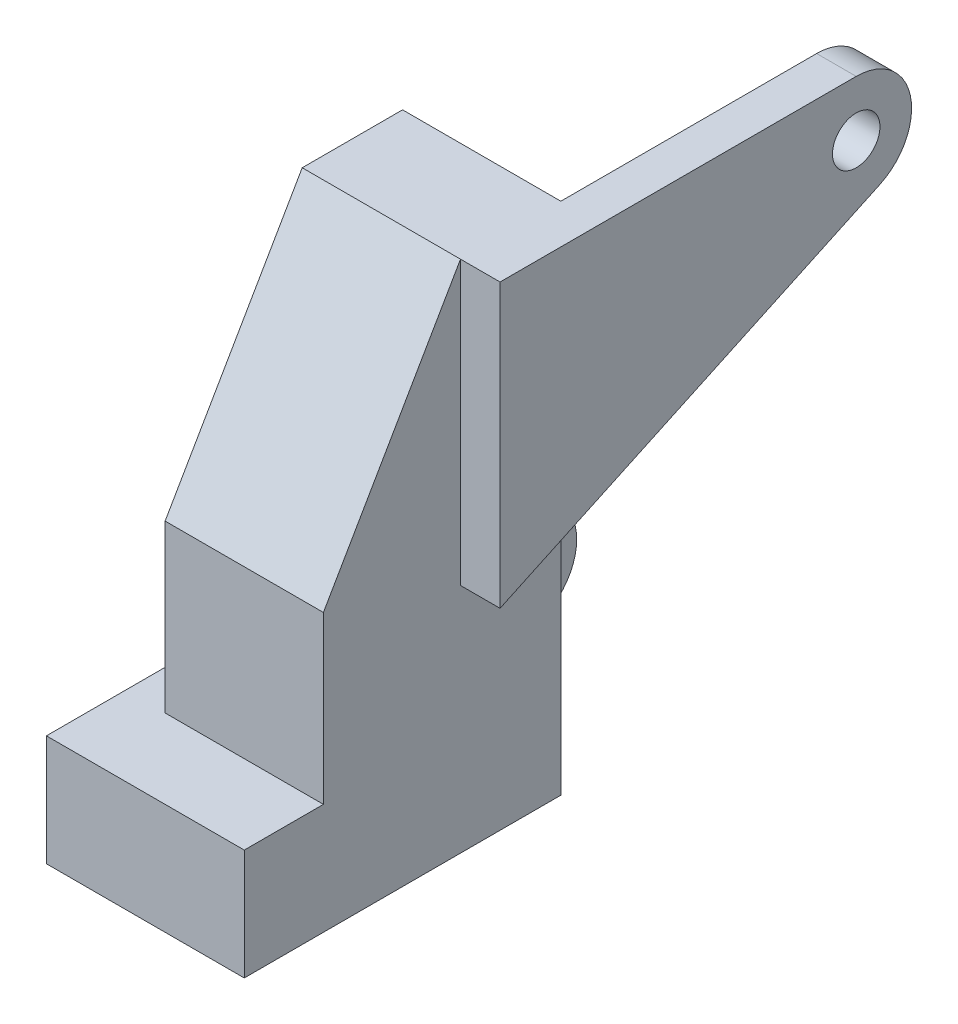
ISO-10303-21;
HEADER;
FILE_DESCRIPTION(('STEP AP214'),'2;1');
FILE_NAME('part.step','',(''),(''),'','','');
FILE_SCHEMA(('AUTOMOTIVE_DESIGN { 1 0 10303 214 1 1 1 1 }'));
ENDSEC;
DATA;
#1=APPLICATION_CONTEXT('core data for automotive mechanical design processes');
#2=APPLICATION_PROTOCOL_DEFINITION('international standard','automotive_design',2000,#1);
#3=PRODUCT_CONTEXT('',#1,'mechanical');
#4=PRODUCT('Part','Part','',(#3));
#5=PRODUCT_RELATED_PRODUCT_CATEGORY('part','',(#4));
#6=PRODUCT_DEFINITION_FORMATION('','',#4);
#7=PRODUCT_DEFINITION_CONTEXT('part definition',#1,'design');
#8=PRODUCT_DEFINITION('design','',#6,#7);
#9=PRODUCT_DEFINITION_SHAPE('','',#8);
#10=(LENGTH_UNIT() NAMED_UNIT(*) SI_UNIT(.MILLI.,.METRE.));
#11=(NAMED_UNIT(*) PLANE_ANGLE_UNIT() SI_UNIT($,.RADIAN.));
#12=(NAMED_UNIT(*) SI_UNIT($,.STERADIAN.) SOLID_ANGLE_UNIT());
#13=UNCERTAINTY_MEASURE_WITH_UNIT(LENGTH_MEASURE(1.E-05),#10,'distance_accuracy_value','');
#14=(GEOMETRIC_REPRESENTATION_CONTEXT(3) GLOBAL_UNCERTAINTY_ASSIGNED_CONTEXT((#13)) GLOBAL_UNIT_ASSIGNED_CONTEXT((#10,
#11,#12)) REPRESENTATION_CONTEXT('',''));
#15=CARTESIAN_POINT('',(0.,0.,0.));
#16=DIRECTION('',(0.,0.,1.));
#17=DIRECTION('',(1.,0.,0.));
#18=AXIS2_PLACEMENT_3D('',#15,#16,#17);
#19=CARTESIAN_POINT('',(9.99999999999999,32.5,40.));
#20=DIRECTION('',(-1.,0.,0.));
#21=DIRECTION('',(0.,-1.,0.));
#22=AXIS2_PLACEMENT_3D('',#19,#20,#21);
#23=PLANE('',#22);
#24=DIRECTION('',(0.,0.422618261740704,-0.906307787036648));
#25=VECTOR('',#24,1.);
#26=CARTESIAN_POINT('',(10.,-3.20749004971267,12.6794919243115));
#27=LINE('',#26,#25);
#28=CARTESIAN_POINT('',(10.,-3.20749004971267,12.6794919243115));
#29=VERTEX_POINT('',#28);
#30=CARTESIAN_POINT('',(10.,2.7050541361083,0.));
#31=VERTEX_POINT('',#30);
#32=EDGE_CURVE('E483',#29,#31,#27,.T.);
#33=ORIENTED_EDGE('',*,*,#32,.F.);
#34=DIRECTION('',(0.,-1.,0.));
#35=VECTOR('',#34,1.);
#36=CARTESIAN_POINT('',(9.99999999999999,32.5,12.6794919243115));
#37=LINE('',#36,#35);
#38=CARTESIAN_POINT('',(9.99999999999999,32.5,12.6794919243115));
#39=VERTEX_POINT('',#38);
#40=EDGE_CURVE('E481',#39,#29,#37,.T.);
#41=ORIENTED_EDGE('',*,*,#40,.F.);
#42=DIRECTION('',(0.,0.866025403784442,-0.499999999999995));
#43=VECTOR('',#42,1.);
#44=CARTESIAN_POINT('',(9.99999999999999,32.5,12.6794919243115));
#45=LINE('',#44,#43);
#46=CARTESIAN_POINT('',(10.,2.5,30.));
#47=VERTEX_POINT('',#46);
#48=EDGE_CURVE('E208',#47,#39,#45,.T.);
#49=ORIENTED_EDGE('',*,*,#48,.F.);
#50=DIRECTION('',(0.,1.,0.));
#51=VECTOR('',#50,1.);
#52=CARTESIAN_POINT('',(10.,-18.5,30.));
#53=LINE('',#52,#51);
#54=CARTESIAN_POINT('',(10.,-18.5,30.));
#55=VERTEX_POINT('',#54);
#56=EDGE_CURVE('E204',#55,#47,#53,.T.);
#57=ORIENTED_EDGE('',*,*,#56,.F.);
#58=DIRECTION('',(0.,0.,1.));
#59=VECTOR('',#58,1.);
#60=CARTESIAN_POINT('',(10.,-18.5,-15.));
#61=LINE('',#60,#59);
#62=CARTESIAN_POINT('',(10.,-18.5,40.));
#63=VERTEX_POINT('',#62);
#64=EDGE_CURVE('E11',#55,#63,#61,.T.);
#65=ORIENTED_EDGE('',*,*,#64,.T.);
#66=DIRECTION('',(0.,-1.,0.));
#67=VECTOR('',#66,1.);
#68=CARTESIAN_POINT('',(10.,-18.5,40.));
#69=LINE('',#68,#67);
#70=CARTESIAN_POINT('',(10.,-32.5,40.));
#71=VERTEX_POINT('',#70);
#72=EDGE_CURVE('E174',#63,#71,#69,.T.);
#73=ORIENTED_EDGE('',*,*,#72,.T.);
#74=DIRECTION('',(0.,0.,-1.));
#75=VECTOR('',#74,1.);
#76=CARTESIAN_POINT('',(10.,-32.5,40.));
#77=LINE('',#76,#75);
#78=CARTESIAN_POINT('',(10.,-32.5,0.));
#79=VERTEX_POINT('',#78);
#80=EDGE_CURVE('E178',#71,#79,#77,.T.);
#81=ORIENTED_EDGE('',*,*,#80,.T.);
#82=DIRECTION('',(0.,1.,0.));
#83=VECTOR('',#82,1.);
#84=CARTESIAN_POINT('',(9.99999999999999,32.5,0.));
#85=LINE('',#84,#83);
#86=EDGE_CURVE('E233',#79,#31,#85,.T.);
#87=ORIENTED_EDGE('',*,*,#86,.T.);
#88=EDGE_LOOP('',(#33,#41,#49,#57,#65,#73,#81,#87));
#89=FACE_BOUND('',#88,.T.);
#90=ADVANCED_FACE('F39',(#89),#23,.F.);
#91=CARTESIAN_POINT('',(-9.99999999999999,-32.5,40.));
#92=DIRECTION('',(0.,1.,0.));
#93=DIRECTION('',(0.,0.,1.));
#94=AXIS2_PLACEMENT_3D('',#91,#92,#93);
#95=PLANE('',#94);
#96=ORIENTED_EDGE('',*,*,#80,.F.);
#97=DIRECTION('',(1.,0.,0.));
#98=VECTOR('',#97,1.);
#99=CARTESIAN_POINT('',(-9.99999999999999,-32.5,40.));
#100=LINE('',#99,#98);
#101=CARTESIAN_POINT('',(-15.,-32.5,40.));
#102=VERTEX_POINT('',#101);
#103=EDGE_CURVE('E224',#102,#71,#100,.T.);
#104=ORIENTED_EDGE('',*,*,#103,.F.);
#105=DIRECTION('',(0.,0.,-1.));
#106=VECTOR('',#105,1.);
#107=CARTESIAN_POINT('',(-15.,-32.5,40.));
#108=LINE('',#107,#106);
#109=CARTESIAN_POINT('',(-15.,-32.5,-15.));
#110=VERTEX_POINT('',#109);
#111=EDGE_CURVE('E192',#102,#110,#108,.T.);
#112=ORIENTED_EDGE('',*,*,#111,.T.);
#113=DIRECTION('',(1.,0.,0.));
#114=VECTOR('',#113,1.);
#115=CARTESIAN_POINT('',(-15.,-32.5,-15.));
#116=LINE('',#115,#114);
#117=CARTESIAN_POINT('',(-10.,-32.5,-15.));
#118=VERTEX_POINT('',#117);
#119=EDGE_CURVE('E191',#110,#118,#116,.T.);
#120=ORIENTED_EDGE('',*,*,#119,.T.);
#121=DIRECTION('',(0.,0.,-1.));
#122=VECTOR('',#121,1.);
#123=CARTESIAN_POINT('',(-10.,-32.5,40.));
#124=LINE('',#123,#122);
#125=CARTESIAN_POINT('',(-9.99999999999999,-32.5,0.));
#126=VERTEX_POINT('',#125);
#127=EDGE_CURVE('E184',#126,#118,#124,.T.);
#128=ORIENTED_EDGE('',*,*,#127,.F.);
#129=DIRECTION('',(1.,0.,0.));
#130=VECTOR('',#129,1.);
#131=CARTESIAN_POINT('',(-9.99999999999999,-32.5,0.));
#132=LINE('',#131,#130);
#133=EDGE_CURVE('E225',#126,#79,#132,.T.);
#134=ORIENTED_EDGE('',*,*,#133,.T.);
#135=EDGE_LOOP('',(#96,#104,#112,#120,#128,#134));
#136=FACE_BOUND('',#135,.T.);
#137=ADVANCED_FACE('F247',(#136),#95,.F.);
#138=CARTESIAN_POINT('',(-10.,-18.5,30.));
#139=DIRECTION('',(0.,-1.,0.));
#140=DIRECTION('',(1.,0.,0.));
#141=AXIS2_PLACEMENT_3D('',#138,#139,#140);
#142=PLANE('',#141);
#143=ORIENTED_EDGE('',*,*,#64,.F.);
#144=DIRECTION('',(1.,0.,0.));
#145=VECTOR('',#144,1.);
#146=CARTESIAN_POINT('',(-10.,-18.5,30.));
#147=LINE('',#146,#145);
#148=CARTESIAN_POINT('',(-10.,-18.5,30.));
#149=VERTEX_POINT('',#148);
#150=EDGE_CURVE('E211',#149,#55,#147,.T.);
#151=ORIENTED_EDGE('',*,*,#150,.F.);
#152=DIRECTION('',(0.,0.,1.));
#153=VECTOR('',#152,1.);
#154=CARTESIAN_POINT('',(-10.,-18.5,40.));
#155=LINE('',#154,#153);
#156=CARTESIAN_POINT('',(-10.,-18.5,0.));
#157=VERTEX_POINT('',#156);
#158=EDGE_CURVE('E50',#157,#149,#155,.T.);
#159=ORIENTED_EDGE('',*,*,#158,.F.);
#160=CARTESIAN_POINT('',(-10.,-18.5,-15.));
#161=VERTEX_POINT('',#160);
#162=EDGE_CURVE('E179',#161,#157,#155,.T.);
#163=ORIENTED_EDGE('',*,*,#162,.F.);
#164=DIRECTION('',(1.,0.,0.));
#165=VECTOR('',#164,1.);
#166=CARTESIAN_POINT('',(-15.,-18.5,-15.));
#167=LINE('',#166,#165);
#168=CARTESIAN_POINT('',(-15.,-18.5,-15.));
#169=VERTEX_POINT('',#168);
#170=EDGE_CURVE('E202',#169,#161,#167,.T.);
#171=ORIENTED_EDGE('',*,*,#170,.F.);
#172=DIRECTION('',(0.,0.,1.));
#173=VECTOR('',#172,1.);
#174=CARTESIAN_POINT('',(-15.,-18.5,40.));
#175=LINE('',#174,#173);
#176=CARTESIAN_POINT('',(-15.,-18.5,40.));
#177=VERTEX_POINT('',#176);
#178=EDGE_CURVE('E183',#169,#177,#175,.T.);
#179=ORIENTED_EDGE('',*,*,#178,.T.);
#180=DIRECTION('',(1.,0.,0.));
#181=VECTOR('',#180,1.);
#182=CARTESIAN_POINT('',(-10.,-18.5,40.));
#183=LINE('',#182,#181);
#184=EDGE_CURVE('E214',#177,#63,#183,.T.);
#185=ORIENTED_EDGE('',*,*,#184,.T.);
#186=EDGE_LOOP('',(#143,#151,#159,#163,#171,#179,#185));
#187=FACE_BOUND('',#186,.T.);
#188=ADVANCED_FACE('F257',(#187),#142,.F.);
#189=CARTESIAN_POINT('',(-10.,32.5,40.));
#190=DIRECTION('',(0.,-1.,0.));
#191=DIRECTION('',(0.,0.,-1.));
#192=AXIS2_PLACEMENT_3D('',#189,#190,#191);
#193=PLANE('',#192);
#194=DIRECTION('',(0.,0.,-1.));
#195=VECTOR('',#194,1.);
#196=CARTESIAN_POINT('',(-10.,32.5,40.));
#197=LINE('',#196,#195);
#198=CARTESIAN_POINT('',(-10.,32.5,12.6794919243115));
#199=VERTEX_POINT('',#198);
#200=CARTESIAN_POINT('',(-10.,32.5,0.));
#201=VERTEX_POINT('',#200);
#202=EDGE_CURVE('E228',#199,#201,#197,.T.);
#203=ORIENTED_EDGE('',*,*,#202,.F.);
#204=DIRECTION('',(1.,0.,0.));
#205=VECTOR('',#204,1.);
#206=CARTESIAN_POINT('',(-10.,32.5,12.6794919243115));
#207=LINE('',#206,#205);
#208=EDGE_CURVE('E165',#199,#39,#207,.T.);
#209=ORIENTED_EDGE('',*,*,#208,.T.);
#210=DIRECTION('',(-1.,0.,0.));
#211=VECTOR('',#210,1.);
#212=CARTESIAN_POINT('',(15.,32.5,12.6794919243115));
#213=LINE('',#212,#211);
#214=CARTESIAN_POINT('',(15.,32.5,12.6794919243115));
#215=VERTEX_POINT('',#214);
#216=EDGE_CURVE('E141',#215,#39,#213,.T.);
#217=ORIENTED_EDGE('',*,*,#216,.F.);
#218=DIRECTION('',(0.,0.,1.));
#219=VECTOR('',#218,1.);
#220=CARTESIAN_POINT('',(15.,32.5,12.6794919243115));
#221=LINE('',#220,#219);
#222=CARTESIAN_POINT('',(15.,32.5,-32.3205080756885));
#223=VERTEX_POINT('',#222);
#224=EDGE_CURVE('E146',#223,#215,#221,.T.);
#225=ORIENTED_EDGE('',*,*,#224,.F.);
#226=DIRECTION('',(-1.,0.,0.));
#227=VECTOR('',#226,1.);
#228=CARTESIAN_POINT('',(15.,32.5,-32.3205080756885));
#229=LINE('',#228,#227);
#230=CARTESIAN_POINT('',(9.99999999999999,32.5,-32.3205080756885));
#231=VERTEX_POINT('',#230);
#232=EDGE_CURVE('E478',#223,#231,#229,.T.);
#233=ORIENTED_EDGE('',*,*,#232,.T.);
#234=DIRECTION('',(0.,0.,1.));
#235=VECTOR('',#234,1.);
#236=CARTESIAN_POINT('',(9.99999999999999,32.5,12.6794919243115));
#237=LINE('',#236,#235);
#238=CARTESIAN_POINT('',(9.99999999999999,32.5,0.));
#239=VERTEX_POINT('',#238);
#240=EDGE_CURVE('E474',#231,#239,#237,.T.);
#241=ORIENTED_EDGE('',*,*,#240,.T.);
#242=DIRECTION('',(-1.,0.,0.));
#243=VECTOR('',#242,1.);
#244=CARTESIAN_POINT('',(-10.,32.5,0.));
#245=LINE('',#244,#243);
#246=EDGE_CURVE('E226',#239,#201,#245,.T.);
#247=ORIENTED_EDGE('',*,*,#246,.T.);
#248=EDGE_LOOP('',(#203,#209,#217,#225,#233,#241,#247));
#249=FACE_BOUND('',#248,.T.);
#250=ADVANCED_FACE('F161',(#249),#193,.F.);
#251=CARTESIAN_POINT('',(-10.,32.5,40.));
#252=DIRECTION('',(1.,0.,0.));
#253=DIRECTION('',(0.,1.,0.));
#254=AXIS2_PLACEMENT_3D('',#251,#252,#253);
#255=PLANE('',#254);
#256=DIRECTION('',(0.,-1.,0.));
#257=VECTOR('',#256,1.);
#258=CARTESIAN_POINT('',(-10.,32.5,0.));
#259=LINE('',#258,#257);
#260=EDGE_CURVE('E219',#201,#157,#259,.T.);
#261=ORIENTED_EDGE('',*,*,#260,.T.);
#262=ORIENTED_EDGE('',*,*,#158,.T.);
#263=DIRECTION('',(0.,1.,0.));
#264=VECTOR('',#263,1.);
#265=CARTESIAN_POINT('',(-10.,-18.5,30.));
#266=LINE('',#265,#264);
#267=CARTESIAN_POINT('',(-10.,2.50000000000002,30.));
#268=VERTEX_POINT('',#267);
#269=EDGE_CURVE('E207',#149,#268,#266,.T.);
#270=ORIENTED_EDGE('',*,*,#269,.T.);
#271=DIRECTION('',(0.,0.866025403784442,-0.499999999999995));
#272=VECTOR('',#271,1.);
#273=CARTESIAN_POINT('',(-10.,32.5,12.6794919243115));
#274=LINE('',#273,#272);
#275=EDGE_CURVE('E209',#268,#199,#274,.T.);
#276=ORIENTED_EDGE('',*,*,#275,.T.);
#277=ORIENTED_EDGE('',*,*,#202,.T.);
#278=EDGE_LOOP('',(#261,#262,#270,#276,#277));
#279=FACE_BOUND('',#278,.T.);
#280=ADVANCED_FACE('F263',(#279),#255,.F.);
#281=CARTESIAN_POINT('',(0.,0.,40.));
#282=DIRECTION('',(0.,0.,1.));
#283=DIRECTION('',(1.,0.,0.));
#284=AXIS2_PLACEMENT_3D('',#281,#282,#283);
#285=PLANE('',#284);
#286=ORIENTED_EDGE('',*,*,#72,.F.);
#287=ORIENTED_EDGE('',*,*,#184,.F.);
#288=DIRECTION('',(0.,-1.,0.));
#289=VECTOR('',#288,1.);
#290=CARTESIAN_POINT('',(-15.,-32.5,40.));
#291=LINE('',#290,#289);
#292=EDGE_CURVE('E181',#177,#102,#291,.T.);
#293=ORIENTED_EDGE('',*,*,#292,.T.);
#294=ORIENTED_EDGE('',*,*,#103,.T.);
#295=EDGE_LOOP('',(#286,#287,#293,#294));
#296=FACE_BOUND('',#295,.T.);
#297=ADVANCED_FACE('F243',(#296),#285,.T.);
#298=CARTESIAN_POINT('',(0.,0.,0.));
#299=DIRECTION('',(0.,0.,1.));
#300=DIRECTION('',(1.,0.,0.));
#301=AXIS2_PLACEMENT_3D('',#298,#299,#300);
#302=PLANE('',#301);
#303=ORIENTED_EDGE('',*,*,#86,.F.);
#304=ORIENTED_EDGE('',*,*,#133,.F.);
#305=EDGE_CURVE('E65',#157,#126,#259,.T.);
#306=ORIENTED_EDGE('',*,*,#305,.F.);
#307=ORIENTED_EDGE('',*,*,#260,.F.);
#308=ORIENTED_EDGE('',*,*,#246,.F.);
#309=EDGE_CURVE('E54',#31,#239,#85,.T.);
#310=ORIENTED_EDGE('',*,*,#309,.F.);
#311=EDGE_LOOP('',(#303,#304,#306,#307,#308,#310));
#312=FACE_BOUND('',#311,.T.);
#313=ADVANCED_FACE('F297',(#312),#302,.F.);
#314=CARTESIAN_POINT('',(-10.,32.5,12.6794919243115));
#315=DIRECTION('',(0.,-0.499999999999995,-0.866025403784442));
#316=DIRECTION('',(0.,0.866025403784442,-0.499999999999995));
#317=AXIS2_PLACEMENT_3D('',#314,#315,#316);
#318=PLANE('',#317);
#319=ORIENTED_EDGE('',*,*,#208,.F.);
#320=ORIENTED_EDGE('',*,*,#275,.F.);
#321=DIRECTION('',(1.,0.,0.));
#322=VECTOR('',#321,1.);
#323=CARTESIAN_POINT('',(-10.,2.50000000000002,30.));
#324=LINE('',#323,#322);
#325=EDGE_CURVE('E220',#268,#47,#324,.T.);
#326=ORIENTED_EDGE('',*,*,#325,.T.);
#327=ORIENTED_EDGE('',*,*,#48,.T.);
#328=EDGE_LOOP('',(#319,#320,#326,#327));
#329=FACE_BOUND('',#328,.T.);
#330=ADVANCED_FACE('F313',(#329),#318,.F.);
#331=CARTESIAN_POINT('',(-10.,-18.5,30.));
#332=DIRECTION('',(0.,0.,-1.));
#333=DIRECTION('',(0.,1.,0.));
#334=AXIS2_PLACEMENT_3D('',#331,#332,#333);
#335=PLANE('',#334);
#336=ORIENTED_EDGE('',*,*,#325,.F.);
#337=ORIENTED_EDGE('',*,*,#269,.F.);
#338=ORIENTED_EDGE('',*,*,#150,.T.);
#339=ORIENTED_EDGE('',*,*,#56,.T.);
#340=EDGE_LOOP('',(#336,#337,#338,#339));
#341=FACE_BOUND('',#340,.T.);
#342=ADVANCED_FACE('F261',(#341),#335,.F.);
#343=CARTESIAN_POINT('',(-10.,-25.5,-15.));
#344=DIRECTION('',(-1.,0.,0.));
#345=DIRECTION('',(0.,1.,0.));
#346=AXIS2_PLACEMENT_3D('',#343,#344,#345);
#347=PLANE('',#346);
#348=CARTESIAN_POINT('',(-10.,-25.5,-15.));
#349=DIRECTION('',(1.,0.,0.));
#350=DIRECTION('',(0.,1.,0.));
#351=AXIS2_PLACEMENT_3D('',#348,#349,#350);
#352=CIRCLE('',#351,3.5);
#353=CARTESIAN_POINT('',(-10.,-22.,-15.));
#354=VERTEX_POINT('',#353);
#355=EDGE_CURVE('E164',#354,#354,#352,.T.);
#356=ORIENTED_EDGE('',*,*,#355,.F.);
#357=EDGE_LOOP('',(#356));
#358=FACE_BOUND('',#357,.T.);
#359=ORIENTED_EDGE('',*,*,#162,.T.);
#360=ORIENTED_EDGE('',*,*,#305,.T.);
#361=ORIENTED_EDGE('',*,*,#127,.T.);
#362=CARTESIAN_POINT('',(-10.,-25.5,-15.));
#363=DIRECTION('',(1.,0.,0.));
#364=DIRECTION('',(0.,1.,0.));
#365=AXIS2_PLACEMENT_3D('',#362,#363,#364);
#366=CIRCLE('',#365,7.);
#367=EDGE_CURVE('E200',#118,#161,#366,.T.);
#368=ORIENTED_EDGE('',*,*,#367,.T.);
#369=EDGE_LOOP('',(#359,#360,#361,#368));
#370=FACE_BOUND('',#369,.T.);
#371=ADVANCED_FACE('F266',(#358,#370),#347,.F.);
#372=CARTESIAN_POINT('',(-15.,-25.5,-15.));
#373=DIRECTION('',(1.,0.,0.));
#374=DIRECTION('',(0.,1.,0.));
#375=AXIS2_PLACEMENT_3D('',#372,#373,#374);
#376=CYLINDRICAL_SURFACE('',#375,7.);
#377=ORIENTED_EDGE('',*,*,#367,.F.);
#378=ORIENTED_EDGE('',*,*,#119,.F.);
#379=CARTESIAN_POINT('',(-15.,-25.5,-15.));
#380=DIRECTION('',(1.,0.,0.));
#381=DIRECTION('',(0.,1.,0.));
#382=AXIS2_PLACEMENT_3D('',#379,#380,#381);
#383=CIRCLE('',#382,7.);
#384=EDGE_CURVE('E189',#110,#169,#383,.T.);
#385=ORIENTED_EDGE('',*,*,#384,.T.);
#386=ORIENTED_EDGE('',*,*,#170,.T.);
#387=EDGE_LOOP('',(#377,#378,#385,#386));
#388=FACE_BOUND('',#387,.T.);
#389=ADVANCED_FACE('F268',(#388),#376,.T.);
#390=CARTESIAN_POINT('',(-15.,-25.5,-15.));
#391=DIRECTION('',(-1.,0.,0.));
#392=DIRECTION('',(0.,1.,0.));
#393=AXIS2_PLACEMENT_3D('',#390,#391,#392);
#394=PLANE('',#393);
#395=CARTESIAN_POINT('',(-15.,-25.5,-15.));
#396=DIRECTION('',(1.,0.,0.));
#397=DIRECTION('',(0.,1.,0.));
#398=AXIS2_PLACEMENT_3D('',#395,#396,#397);
#399=CIRCLE('',#398,3.5);
#400=CARTESIAN_POINT('',(-15.,-22.,-15.));
#401=VERTEX_POINT('',#400);
#402=EDGE_CURVE('E166',#401,#401,#399,.T.);
#403=ORIENTED_EDGE('',*,*,#402,.T.);
#404=EDGE_LOOP('',(#403));
#405=FACE_BOUND('',#404,.T.);
#406=ORIENTED_EDGE('',*,*,#292,.F.);
#407=ORIENTED_EDGE('',*,*,#178,.F.);
#408=ORIENTED_EDGE('',*,*,#384,.F.);
#409=ORIENTED_EDGE('',*,*,#111,.F.);
#410=EDGE_LOOP('',(#406,#407,#408,#409));
#411=FACE_BOUND('',#410,.T.);
#412=ADVANCED_FACE('F271',(#405,#411),#394,.T.);
#413=CARTESIAN_POINT('',(-15.,-25.5,-15.));
#414=DIRECTION('',(1.,0.,0.));
#415=DIRECTION('',(0.,1.,0.));
#416=AXIS2_PLACEMENT_3D('',#413,#414,#415);
#417=CYLINDRICAL_SURFACE('',#416,3.5);
#418=ORIENTED_EDGE('',*,*,#402,.F.);
#419=EDGE_LOOP('',(#418));
#420=FACE_BOUND('',#419,.T.);
#421=ORIENTED_EDGE('',*,*,#355,.T.);
#422=EDGE_LOOP('',(#421));
#423=FACE_BOUND('',#422,.T.);
#424=ADVANCED_FACE('F273',(#420,#423),#417,.F.);
#425=CARTESIAN_POINT('',(10.,25.5,-32.3205080756885));
#426=DIRECTION('',(1.,0.,0.));
#427=DIRECTION('',(0.,1.,0.));
#428=AXIS2_PLACEMENT_3D('',#425,#426,#427);
#429=PLANE('',#428);
#430=CARTESIAN_POINT('',(10.,25.5,-32.3205080756885));
#431=DIRECTION('',(1.,0.,0.));
#432=DIRECTION('',(0.,1.,0.));
#433=AXIS2_PLACEMENT_3D('',#430,#431,#432);
#434=CIRCLE('',#433,3.);
#435=CARTESIAN_POINT('',(10.,28.5,-32.3205080756885));
#436=VERTEX_POINT('',#435);
#437=EDGE_CURVE('E472',#436,#436,#434,.T.);
#438=ORIENTED_EDGE('',*,*,#437,.T.);
#439=EDGE_LOOP('',(#438));
#440=FACE_BOUND('',#439,.T.);
#441=CARTESIAN_POINT('',(10.,19.1558454907435,-35.2788359078735));
#442=VERTEX_POINT('',#441);
#443=EDGE_CURVE('E482',#31,#442,#27,.T.);
#444=ORIENTED_EDGE('',*,*,#443,.F.);
#445=ORIENTED_EDGE('',*,*,#309,.T.);
#446=ORIENTED_EDGE('',*,*,#240,.F.);
#447=CARTESIAN_POINT('',(10.,25.5,-32.3205080756885));
#448=DIRECTION('',(1.,0.,0.));
#449=DIRECTION('',(0.,1.,0.));
#450=AXIS2_PLACEMENT_3D('',#447,#448,#449);
#451=CIRCLE('',#450,7.);
#452=EDGE_CURVE('E158',#442,#231,#451,.T.);
#453=ORIENTED_EDGE('',*,*,#452,.F.);
#454=EDGE_LOOP('',(#444,#445,#446,#453));
#455=FACE_BOUND('',#454,.T.);
#456=ADVANCED_FACE('F285',(#440,#455),#429,.F.);
#457=CARTESIAN_POINT('',(15.,25.5,-32.3205080756885));
#458=DIRECTION('',(1.,0.,0.));
#459=DIRECTION('',(0.,1.,0.));
#460=AXIS2_PLACEMENT_3D('',#457,#458,#459);
#461=PLANE('',#460);
#462=ORIENTED_EDGE('',*,*,#224,.T.);
#463=DIRECTION('',(0.,-1.,0.));
#464=VECTOR('',#463,1.);
#465=CARTESIAN_POINT('',(15.,32.5,12.6794919243115));
#466=LINE('',#465,#464);
#467=CARTESIAN_POINT('',(15.,-3.20749004971267,12.6794919243115));
#468=VERTEX_POINT('',#467);
#469=EDGE_CURVE('E137',#215,#468,#466,.T.);
#470=ORIENTED_EDGE('',*,*,#469,.T.);
#471=DIRECTION('',(0.,0.422618261740704,-0.906307787036648));
#472=VECTOR('',#471,1.);
#473=CARTESIAN_POINT('',(15.,-3.20749004971267,12.6794919243115));
#474=LINE('',#473,#472);
#475=CARTESIAN_POINT('',(15.,19.1558454907435,-35.2788359078735));
#476=VERTEX_POINT('',#475);
#477=EDGE_CURVE('E149',#468,#476,#474,.T.);
#478=ORIENTED_EDGE('',*,*,#477,.T.);
#479=CARTESIAN_POINT('',(15.,25.5,-32.3205080756885));
#480=DIRECTION('',(1.,0.,0.));
#481=DIRECTION('',(0.,1.,0.));
#482=AXIS2_PLACEMENT_3D('',#479,#480,#481);
#483=CIRCLE('',#482,7.);
#484=EDGE_CURVE('E154',#476,#223,#483,.T.);
#485=ORIENTED_EDGE('',*,*,#484,.T.);
#486=EDGE_LOOP('',(#462,#470,#478,#485));
#487=FACE_BOUND('',#486,.T.);
#488=CARTESIAN_POINT('',(15.,25.5,-32.3205080756885));
#489=DIRECTION('',(1.,0.,0.));
#490=DIRECTION('',(0.,1.,0.));
#491=AXIS2_PLACEMENT_3D('',#488,#489,#490);
#492=CIRCLE('',#491,3.);
#493=CARTESIAN_POINT('',(15.,28.5,-32.3205080756885));
#494=VERTEX_POINT('',#493);
#495=EDGE_CURVE('E466',#494,#494,#492,.T.);
#496=ORIENTED_EDGE('',*,*,#495,.F.);
#497=EDGE_LOOP('',(#496));
#498=FACE_BOUND('',#497,.T.);
#499=ADVANCED_FACE('F155',(#487,#498),#461,.T.);
#500=CARTESIAN_POINT('',(15.,32.5,12.6794919243115));
#501=DIRECTION('',(0.,0.,-1.));
#502=DIRECTION('',(0.,1.,0.));
#503=AXIS2_PLACEMENT_3D('',#500,#501,#502);
#504=PLANE('',#503);
#505=ORIENTED_EDGE('',*,*,#40,.T.);
#506=DIRECTION('',(-1.,0.,0.));
#507=VECTOR('',#506,1.);
#508=CARTESIAN_POINT('',(15.,-3.20749004971267,12.6794919243115));
#509=LINE('',#508,#507);
#510=EDGE_CURVE('E143',#468,#29,#509,.T.);
#511=ORIENTED_EDGE('',*,*,#510,.F.);
#512=ORIENTED_EDGE('',*,*,#469,.F.);
#513=ORIENTED_EDGE('',*,*,#216,.T.);
#514=EDGE_LOOP('',(#505,#511,#512,#513));
#515=FACE_BOUND('',#514,.T.);
#516=ADVANCED_FACE('F142',(#515),#504,.F.);
#517=CARTESIAN_POINT('',(15.,-3.20749004971267,12.6794919243115));
#518=DIRECTION('',(0.,0.906307787036648,0.422618261740704));
#519=DIRECTION('',(0.,-0.422618261740704,0.906307787036648));
#520=AXIS2_PLACEMENT_3D('',#517,#518,#519);
#521=PLANE('',#520);
#522=ORIENTED_EDGE('',*,*,#32,.T.);
#523=ORIENTED_EDGE('',*,*,#443,.T.);
#524=DIRECTION('',(-1.,0.,0.));
#525=VECTOR('',#524,1.);
#526=CARTESIAN_POINT('',(15.,19.1558454907435,-35.2788359078735));
#527=LINE('',#526,#525);
#528=EDGE_CURVE('E167',#476,#442,#527,.T.);
#529=ORIENTED_EDGE('',*,*,#528,.F.);
#530=ORIENTED_EDGE('',*,*,#477,.F.);
#531=ORIENTED_EDGE('',*,*,#510,.T.);
#532=EDGE_LOOP('',(#522,#523,#529,#530,#531));
#533=FACE_BOUND('',#532,.T.);
#534=ADVANCED_FACE('F343',(#533),#521,.F.);
#535=CARTESIAN_POINT('',(15.,25.5,-32.3205080756885));
#536=DIRECTION('',(-1.,0.,0.));
#537=DIRECTION('',(0.,-1.,0.));
#538=AXIS2_PLACEMENT_3D('',#535,#536,#537);
#539=CYLINDRICAL_SURFACE('',#538,7.);
#540=ORIENTED_EDGE('',*,*,#452,.T.);
#541=ORIENTED_EDGE('',*,*,#232,.F.);
#542=ORIENTED_EDGE('',*,*,#484,.F.);
#543=ORIENTED_EDGE('',*,*,#528,.T.);
#544=EDGE_LOOP('',(#540,#541,#542,#543));
#545=FACE_BOUND('',#544,.T.);
#546=ADVANCED_FACE('F352',(#545),#539,.T.);
#547=CARTESIAN_POINT('',(15.,25.5,-32.3205080756885));
#548=DIRECTION('',(-1.,0.,0.));
#549=DIRECTION('',(0.,-1.,0.));
#550=AXIS2_PLACEMENT_3D('',#547,#548,#549);
#551=CYLINDRICAL_SURFACE('',#550,3.);
#552=ORIENTED_EDGE('',*,*,#495,.T.);
#553=EDGE_LOOP('',(#552));
#554=FACE_BOUND('',#553,.T.);
#555=ORIENTED_EDGE('',*,*,#437,.F.);
#556=EDGE_LOOP('',(#555));
#557=FACE_BOUND('',#556,.T.);
#558=ADVANCED_FACE('F365',(#554,#557),#551,.F.);
#559=CLOSED_SHELL('',(#90,#137,#188,#250,#280,#297,#313,#330,#342,#371,#389,#412,#424,#456,#499,
#516,#534,#546,#558));
#560=MANIFOLD_SOLID_BREP('B2',#559);
#561=ADVANCED_BREP_SHAPE_REPRESENTATION('',(#18,#560),#14);
#562=SHAPE_DEFINITION_REPRESENTATION(#9,#561);
ENDSEC;
END-ISO-10303-21;
